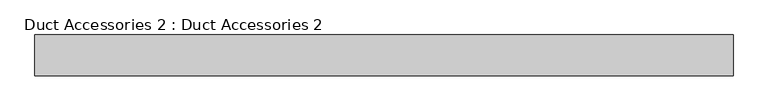
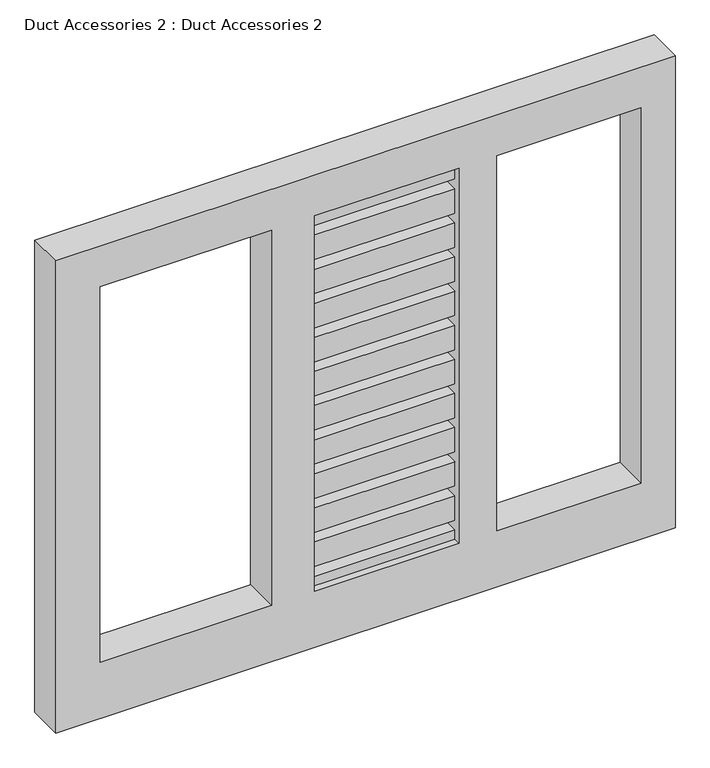
"""IFC4 building model written with IfcOpenShell, lengths in millimetres: damper geometry, Duct Accessories 2 : Duct Accessories 2."""

from ifc_helpers import new_model, si_unit, frame, origin, place, context, project, spatial, polyline, outline, extrude, faceted_brep, source, transform, mapped, element, save


def duct_accessories_2_duct_accessories_2_621c73fd(model_context):
    return source(origin(), model_context, "Body", "SolidModel", [
        extrude(outline(polyline([(-4990.9296146, 8704.654407), (-4990.9296146, 5351.854407), (-5235.4994609, 5351.854407), (-5235.4994609, 5436.5437565), (-5048.1296146, 5436.5437565), (-5048.1296146, 5523.4610067), (-5235.4994609, 5523.4610067), (-5235.4994609, 5741.3437565), (-5048.1296146, 5741.3437565), (-5048.1296146, 5828.2610067), (-5235.4994609, 5828.2610067), (-5235.4994609, 6046.1437565), (-5048.1296146, 6046.1437565), (-5048.1296146, 6133.0610067), (-5235.4994609, 6133.0610067), (-5235.4994609, 6350.9437565), (-5048.1296146, 6350.9437565), (-5048.1296146, 6437.8610067), (-5235.4994609, 6437.8610067), (-5235.4994609, 6655.7437565), (-5048.1296146, 6655.7437565), (-5048.1296146, 6742.6610067), (-5235.4994609, 6742.6610067), (-5235.4994609, 6960.5437565), (-5048.1296146, 6960.5437565), (-5048.1296146, 7047.4610067), (-5235.4994609, 7047.4610067), (-5235.4994609, 7265.3437565), (-5048.1296146, 7265.3437565), (-5048.1296146, 7352.2610067), (-5235.4994609, 7352.2610067), (-5235.4994609, 7570.1437565), (-5048.1296146, 7570.1437565), (-5048.1296146, 7657.0610067), (-5235.4994609, 7657.0610067), (-5235.4994609, 7874.9437565), (-5048.1296146, 7874.9437565), (-5048.1296146, 7961.8610067), (-5235.4994609, 7961.8610067), (-5235.4994609, 8179.7437565), (-5048.1296146, 8179.7437565), (-5048.1296146, 8266.6610067), (-5235.4994609, 8266.6610067), (-5235.4994609, 8484.5437565), (-5048.1296146, 8484.5437565), (-5048.1296146, 8571.4610067), (-5235.4994609, 8571.4610067), (-5235.4994609, 8704.654407), (-4990.9296146, 8704.654407)])), frame((-9385.4667042, 0.0, 0.0), z_axis=(1.0, 0.0, 0.0), x_axis=(0.0, 1.0, 0.0)), (0.0, 0.0, 1.0), 1219.2),
        faceted_brep([(-6337.4667042, -5295.7296146, 9070.24), (-11576.5067042, -5295.7296146, 9070.24), (-11576.5067042, -5295.7296146, 4850.0), (-6337.4667042, -5295.7296146, 4850.0), (-9750.6667042, -5295.7296146, 8704.654407), (-9750.6667042, -5295.7296146, 5351.854407), (-11198.4667042, -5295.7296146, 5351.854407), (-11198.4667042, -5295.7296146, 8704.654407), (-6626.4667042, -5295.7296146, 8704.654407), (-6626.4667042, -5295.7296146, 5351.854407), (-7845.6667042, -5295.7296146, 5351.854407), (-7845.6667042, -5295.7296146, 8704.654407), (-8166.2667042, -5295.7296146, 5351.854407), (-9385.4667042, -5295.7296146, 5351.854407), (-9385.4667042, -5295.7296146, 5436.5437565), (-9385.4667042, -5295.7296146, 5523.4610067), (-9385.4667042, -5295.7296146, 5741.3437565), (-9385.4667042, -5295.7296146, 5828.2610067), (-9385.4667042, -5295.7296146, 6046.1437565), (-9385.4667042, -5295.7296146, 6133.0610067), (-9385.4667042, -5295.7296146, 6350.9437565), (-9385.4667042, -5295.7296146, 6437.8610067), (-9385.4667042, -5295.7296146, 6655.7437565), (-9385.4667042, -5295.7296146, 6742.6610067), (-9385.4667042, -5295.7296146, 6960.5437565), (-9385.4667042, -5295.7296146, 7047.4610067), (-9385.4667042, -5295.7296146, 7265.3437565), (-9385.4667042, -5295.7296146, 7352.2610067), (-9385.4667042, -5295.7296146, 7570.1437565), (-9385.4667042, -5295.7296146, 7657.0610067), (-9385.4667042, -5295.7296146, 7874.9437565), (-9385.4667042, -5295.7296146, 7961.8610067), (-9385.4667042, -5295.7296146, 8179.7437565), (-9385.4667042, -5295.7296146, 8266.6610067), (-9385.4667042, -5295.7296146, 8484.5437565), (-9385.4667042, -5295.7296146, 8571.4610067), (-9385.4667042, -5295.7296146, 8704.654407), (-8166.2667042, -5295.7296146, 8704.654407), (-8166.2667042, -5295.7296146, 8571.4610067), (-8166.2667042, -5295.7296146, 8484.5437565), (-8166.2667042, -5295.7296146, 8266.6610067), (-8166.2667042, -5295.7296146, 8179.7437565), (-8166.2667042, -5295.7296146, 7961.8610067), (-8166.2667042, -5295.7296146, 7874.9437565), (-8166.2667042, -5295.7296146, 7657.0610067), (-8166.2667042, -5295.7296146, 7570.1437565), (-8166.2667042, -5295.7296146, 7352.2610067), (-8166.2667042, -5295.7296146, 7265.3437565), (-8166.2667042, -5295.7296146, 7047.4610067), (-8166.2667042, -5295.7296146, 6960.5437565), (-8166.2667042, -5295.7296146, 6742.6610067), (-8166.2667042, -5295.7296146, 6655.7437565), (-8166.2667042, -5295.7296146, 6437.8610067), (-8166.2667042, -5295.7296146, 6350.9437565), (-8166.2667042, -5295.7296146, 6133.0610067), (-8166.2667042, -5295.7296146, 6046.1437565), (-8166.2667042, -5295.7296146, 5828.2610067), (-8166.2667042, -5295.7296146, 5741.3437565), (-8166.2667042, -5295.7296146, 5523.4610067), (-8166.2667042, -5295.7296146, 5436.5437565), (-6337.4667042, -4990.9296146, 9070.24), (-6337.4667042, -4990.9296146, 4850.0), (-11576.5067042, -4990.9296146, 4850.0), (-11576.5067042, -4990.9296146, 9070.24), (-9750.6667042, -4990.9296146, 8704.654407), (-11198.4667042, -4990.9296146, 8704.654407), (-11198.4667042, -4990.9296146, 5351.854407), (-9750.6667042, -4990.9296146, 5351.854407), (-6626.4667042, -4990.9296146, 8704.654407), (-7845.6667042, -4990.9296146, 8704.654407), (-7845.6667042, -4990.9296146, 5351.854407), (-6626.4667042, -4990.9296146, 5351.854407), (-8166.2667042, -4990.9296146, 8704.654407), (-9385.4667042, -4990.9296146, 8704.654407), (-9385.4667042, -4990.9296146, 5351.854407), (-8166.2667042, -4990.9296146, 5351.854407)], [[[0, 1, 2, 3], [4, 5, 6, 7], [8, 9, 10, 11], [12, 13, 14, 15, 16, 17, 18, 19, 20, 21, 22, 23, 24, 25, 26, 27, 28, 29, 30, 31, 32, 33, 34, 35, 36, 37, 38, 39, 40, 41, 42, 43, 44, 45, 46, 47, 48, 49, 50, 51, 52, 53, 54, 55, 56, 57, 58, 59]], [[60, 61, 62, 63], [64, 65, 66, 67], [68, 69, 70, 71], [72, 73, 74, 75]], [[1, 0, 60, 63]], [[2, 1, 63, 62]], [[3, 2, 62, 61]], [[0, 3, 61, 60]], [[5, 4, 64, 67]], [[6, 5, 67, 66]], [[7, 6, 66, 65]], [[4, 7, 65, 64]], [[9, 8, 68, 71]], [[10, 9, 71, 70]], [[11, 10, 70, 69]], [[8, 11, 69, 68]], [[72, 75, 12, 59, 58, 57, 56, 55, 54, 53, 52, 51, 50, 49, 48, 47, 46, 45, 44, 43, 42, 41, 40, 39, 38, 37]], [[13, 12, 75, 74]], [[74, 73, 36, 35, 34, 33, 32, 31, 30, 29, 28, 27, 26, 25, 24, 23, 22, 21, 20, 19, 18, 17, 16, 15, 14, 13]], [[37, 36, 73, 72]]]),
    ])


if __name__ == "__main__":
    model = new_model("IFC4")
    model_context = context("Model", 3, world=origin())
    ifc_project = project(units=[si_unit("LENGTHUNIT", "METRE", prefix="MILLI")], contexts=[model_context])
    site = spatial("IfcSite", under=ifc_project)
    building = spatial("IfcBuilding", under=site)
    placement = place(None, origin())
    duct_accessories_2_duct_accessories_2_shape = duct_accessories_2_duct_accessories_2_621c73fd(model_context)
    element("IfcDamper", 1, ObjectType="Duct Accessories 2 : Duct Accessories 2", at=placement, inside=building, context=model_context, shape_type="MappedRepresentation", body=[
        mapped(duct_accessories_2_duct_accessories_2_shape, transform((0.0, 0.0, 0.0), x_axis=(1.0, 0.0, 0.0), y_axis=(0.0, 1.0, 0.0), z_axis=(0.0, 0.0, 1.0))),
    ])
    save(model, "model.ifc")

# Revit data of these elements
# Element 1 (IfcDamper, "Duct Accessories 2 : Duct Accessories 2")
#   Materials on its faces: "GREY"
# Materials
#   "GREY": class "Generic", colour RGB 176 176 176, transparency 0, Cost = 0
